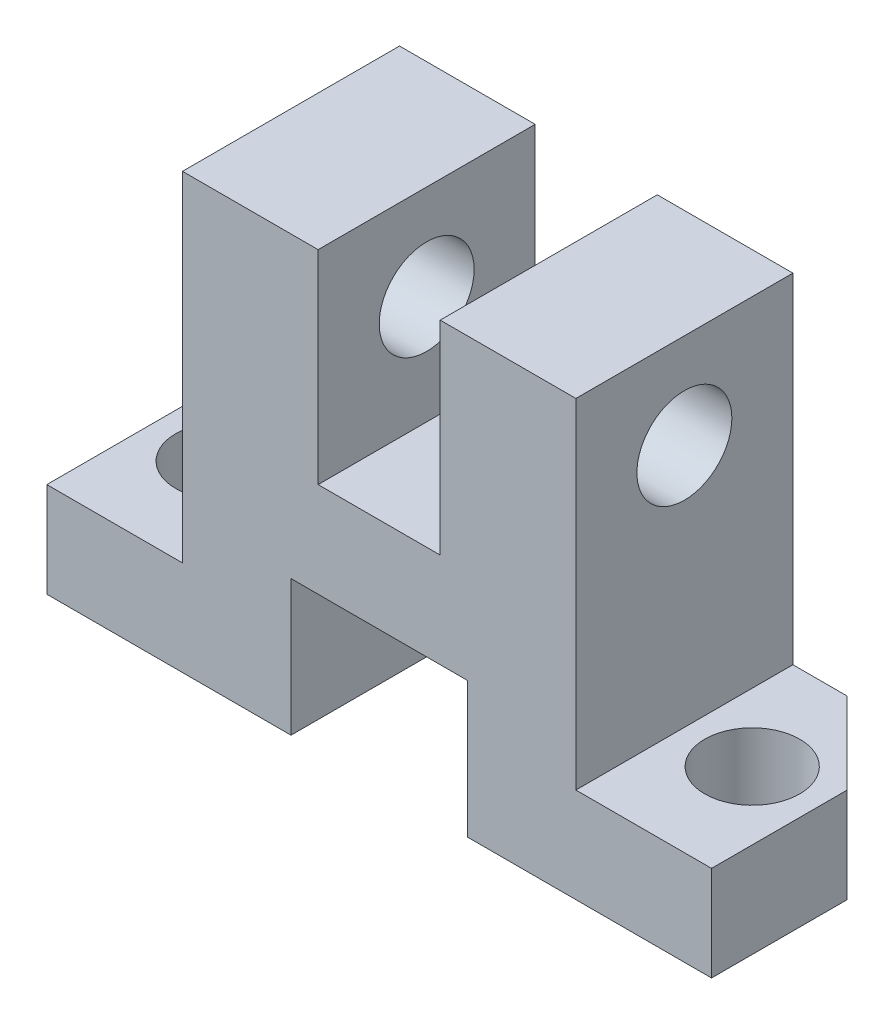
ISO-10303-21;
HEADER;
FILE_DESCRIPTION(('STEP AP214'),'2;1');
FILE_NAME('part.step','',(''),(''),'','','');
FILE_SCHEMA(('AUTOMOTIVE_DESIGN { 1 0 10303 214 1 1 1 1 }'));
ENDSEC;
DATA;
#1=APPLICATION_CONTEXT('core data for automotive mechanical design processes');
#2=APPLICATION_PROTOCOL_DEFINITION('international standard','automotive_design',2000,#1);
#3=PRODUCT_CONTEXT('',#1,'mechanical');
#4=PRODUCT('Part','Part','',(#3));
#5=PRODUCT_RELATED_PRODUCT_CATEGORY('part','',(#4));
#6=PRODUCT_DEFINITION_FORMATION('','',#4);
#7=PRODUCT_DEFINITION_CONTEXT('part definition',#1,'design');
#8=PRODUCT_DEFINITION('design','',#6,#7);
#9=PRODUCT_DEFINITION_SHAPE('','',#8);
#10=(LENGTH_UNIT() NAMED_UNIT(*) SI_UNIT(.MILLI.,.METRE.));
#11=(NAMED_UNIT(*) PLANE_ANGLE_UNIT() SI_UNIT($,.RADIAN.));
#12=(NAMED_UNIT(*) SI_UNIT($,.STERADIAN.) SOLID_ANGLE_UNIT());
#13=UNCERTAINTY_MEASURE_WITH_UNIT(LENGTH_MEASURE(1.E-05),#10,'distance_accuracy_value','');
#14=(GEOMETRIC_REPRESENTATION_CONTEXT(3) GLOBAL_UNCERTAINTY_ASSIGNED_CONTEXT((#13)) GLOBAL_UNIT_ASSIGNED_CONTEXT((#10,
#11,#12)) REPRESENTATION_CONTEXT('',''));
#15=CARTESIAN_POINT('',(0.,0.,0.));
#16=DIRECTION('',(0.,0.,1.));
#17=DIRECTION('',(1.,0.,0.));
#18=AXIS2_PLACEMENT_3D('',#15,#16,#17);
#19=CARTESIAN_POINT('',(14.5,-16.,16.));
#20=DIRECTION('',(-1.,0.,0.));
#21=DIRECTION('',(0.,0.,1.));
#22=AXIS2_PLACEMENT_3D('',#19,#20,#21);
#23=PLANE('',#22);
#24=CARTESIAN_POINT('',(14.5,9.,8.));
#25=DIRECTION('',(1.,0.,0.));
#26=DIRECTION('',(0.,0.,-1.));
#27=AXIS2_PLACEMENT_3D('',#24,#25,#26);
#28=CIRCLE('',#27,3.5);
#29=CARTESIAN_POINT('',(14.5,9.,4.5));
#30=VERTEX_POINT('',#29);
#31=EDGE_CURVE('E234',#30,#30,#28,.T.);
#32=ORIENTED_EDGE('',*,*,#31,.F.);
#33=EDGE_LOOP('',(#32));
#34=FACE_BOUND('',#33,.T.);
#35=DIRECTION('',(0.,0.,1.));
#36=VECTOR('',#35,1.);
#37=CARTESIAN_POINT('',(14.5,-9.00000000000001,0.));
#38=LINE('',#37,#36);
#39=CARTESIAN_POINT('',(14.5,-9.00000000000001,0.));
#40=VERTEX_POINT('',#39);
#41=CARTESIAN_POINT('',(14.5,-9.00000000000001,16.));
#42=VERTEX_POINT('',#41);
#43=EDGE_CURVE('E57',#40,#42,#38,.T.);
#44=ORIENTED_EDGE('',*,*,#43,.F.);
#45=DIRECTION('',(0.,1.,0.));
#46=VECTOR('',#45,1.);
#47=CARTESIAN_POINT('',(14.5,-16.,0.));
#48=LINE('',#47,#46);
#49=CARTESIAN_POINT('',(14.5,16.,0.));
#50=VERTEX_POINT('',#49);
#51=EDGE_CURVE('E287',#40,#50,#48,.T.);
#52=ORIENTED_EDGE('',*,*,#51,.T.);
#53=DIRECTION('',(0.,0.,-1.));
#54=VECTOR('',#53,1.);
#55=CARTESIAN_POINT('',(14.5,16.,16.));
#56=LINE('',#55,#54);
#57=CARTESIAN_POINT('',(14.5,16.,16.));
#58=VERTEX_POINT('',#57);
#59=EDGE_CURVE('E11',#58,#50,#56,.T.);
#60=ORIENTED_EDGE('',*,*,#59,.F.);
#61=DIRECTION('',(0.,1.,0.));
#62=VECTOR('',#61,1.);
#63=CARTESIAN_POINT('',(14.5,-16.,16.));
#64=LINE('',#63,#62);
#65=EDGE_CURVE('E291',#42,#58,#64,.T.);
#66=ORIENTED_EDGE('',*,*,#65,.F.);
#67=EDGE_LOOP('',(#44,#52,#60,#66));
#68=FACE_BOUND('',#67,.T.);
#69=ADVANCED_FACE('F41',(#34,#68),#23,.F.);
#70=CARTESIAN_POINT('',(-14.5,-16.,16.));
#71=DIRECTION('',(1.,0.,0.));
#72=DIRECTION('',(0.,0.,-1.));
#73=AXIS2_PLACEMENT_3D('',#70,#71,#72);
#74=PLANE('',#73);
#75=CARTESIAN_POINT('',(-14.5,9.,8.));
#76=DIRECTION('',(1.,0.,0.));
#77=DIRECTION('',(0.,0.,-1.));
#78=AXIS2_PLACEMENT_3D('',#75,#76,#77);
#79=CIRCLE('',#78,3.5);
#80=CARTESIAN_POINT('',(-14.5,9.,4.5));
#81=VERTEX_POINT('',#80);
#82=EDGE_CURVE('E232',#81,#81,#79,.T.);
#83=ORIENTED_EDGE('',*,*,#82,.T.);
#84=EDGE_LOOP('',(#83));
#85=FACE_BOUND('',#84,.T.);
#86=DIRECTION('',(0.,0.,-1.));
#87=VECTOR('',#86,1.);
#88=CARTESIAN_POINT('',(-14.5,-9.00000000000001,16.));
#89=LINE('',#88,#87);
#90=CARTESIAN_POINT('',(-14.5,-9.00000000000001,16.));
#91=VERTEX_POINT('',#90);
#92=CARTESIAN_POINT('',(-14.5,-9.00000000000001,0.));
#93=VERTEX_POINT('',#92);
#94=EDGE_CURVE('E226',#91,#93,#89,.T.);
#95=ORIENTED_EDGE('',*,*,#94,.F.);
#96=DIRECTION('',(0.,-1.,0.));
#97=VECTOR('',#96,1.);
#98=CARTESIAN_POINT('',(-14.5,-16.,16.));
#99=LINE('',#98,#97);
#100=CARTESIAN_POINT('',(-14.5,16.,16.));
#101=VERTEX_POINT('',#100);
#102=EDGE_CURVE('E297',#101,#91,#99,.T.);
#103=ORIENTED_EDGE('',*,*,#102,.F.);
#104=DIRECTION('',(0.,0.,-1.));
#105=VECTOR('',#104,1.);
#106=CARTESIAN_POINT('',(-14.5,16.,16.));
#107=LINE('',#106,#105);
#108=CARTESIAN_POINT('',(-14.5,16.,0.));
#109=VERTEX_POINT('',#108);
#110=EDGE_CURVE('E47',#101,#109,#107,.T.);
#111=ORIENTED_EDGE('',*,*,#110,.T.);
#112=DIRECTION('',(0.,-1.,0.));
#113=VECTOR('',#112,1.);
#114=CARTESIAN_POINT('',(-14.5,-16.,0.));
#115=LINE('',#114,#113);
#116=EDGE_CURVE('E315',#109,#93,#115,.T.);
#117=ORIENTED_EDGE('',*,*,#116,.T.);
#118=EDGE_LOOP('',(#95,#103,#111,#117));
#119=FACE_BOUND('',#118,.T.);
#120=ADVANCED_FACE('F321',(#85,#119),#74,.F.);
#121=CARTESIAN_POINT('',(-14.5,16.,16.));
#122=DIRECTION('',(0.,-1.,0.));
#123=DIRECTION('',(0.,0.,-1.));
#124=AXIS2_PLACEMENT_3D('',#121,#122,#123);
#125=PLANE('',#124);
#126=DIRECTION('',(-1.,0.,0.));
#127=VECTOR('',#126,1.);
#128=CARTESIAN_POINT('',(-14.5,16.,16.));
#129=LINE('',#128,#127);
#130=CARTESIAN_POINT('',(-4.5,16.,16.));
#131=VERTEX_POINT('',#130);
#132=EDGE_CURVE('E294',#131,#101,#129,.T.);
#133=ORIENTED_EDGE('',*,*,#132,.F.);
#134=DIRECTION('',(0.,0.,1.));
#135=VECTOR('',#134,1.);
#136=CARTESIAN_POINT('',(-4.5,16.,0.));
#137=LINE('',#136,#135);
#138=CARTESIAN_POINT('',(-4.5,16.,0.));
#139=VERTEX_POINT('',#138);
#140=EDGE_CURVE('E256',#139,#131,#137,.T.);
#141=ORIENTED_EDGE('',*,*,#140,.F.);
#142=DIRECTION('',(-1.,0.,0.));
#143=VECTOR('',#142,1.);
#144=CARTESIAN_POINT('',(-14.5,16.,0.));
#145=LINE('',#144,#143);
#146=EDGE_CURVE('E308',#139,#109,#145,.T.);
#147=ORIENTED_EDGE('',*,*,#146,.T.);
#148=ORIENTED_EDGE('',*,*,#110,.F.);
#149=EDGE_LOOP('',(#133,#141,#147,#148));
#150=FACE_BOUND('',#149,.T.);
#151=ADVANCED_FACE('F342',(#150),#125,.F.);
#152=CARTESIAN_POINT('',(-14.5,-16.,16.));
#153=DIRECTION('',(0.,1.,0.));
#154=DIRECTION('',(0.,0.,1.));
#155=AXIS2_PLACEMENT_3D('',#152,#153,#154);
#156=PLANE('',#155);
#157=CARTESIAN_POINT('',(19.5,-16.,8.));
#158=DIRECTION('',(0.,1.,0.));
#159=DIRECTION('',(0.,0.,1.));
#160=AXIS2_PLACEMENT_3D('',#157,#158,#159);
#161=CIRCLE('',#160,3.5);
#162=CARTESIAN_POINT('',(19.5,-16.,11.5));
#163=VERTEX_POINT('',#162);
#164=EDGE_CURVE('E554',#163,#163,#161,.T.);
#165=ORIENTED_EDGE('',*,*,#164,.T.);
#166=EDGE_LOOP('',(#165));
#167=FACE_BOUND('',#166,.T.);
#168=DIRECTION('',(1.,0.,0.));
#169=VECTOR('',#168,1.);
#170=CARTESIAN_POINT('',(-14.5,-16.,16.));
#171=LINE('',#170,#169);
#172=CARTESIAN_POINT('',(6.50000000000001,-16.,16.));
#173=VERTEX_POINT('',#172);
#174=CARTESIAN_POINT('',(24.5,-16.,16.));
#175=VERTEX_POINT('',#174);
#176=EDGE_CURVE('E303',#173,#175,#171,.T.);
#177=ORIENTED_EDGE('',*,*,#176,.F.);
#178=DIRECTION('',(0.,0.,1.));
#179=VECTOR('',#178,1.);
#180=CARTESIAN_POINT('',(6.50000000000001,-16.,0.));
#181=LINE('',#180,#179);
#182=CARTESIAN_POINT('',(6.50000000000001,-16.,0.));
#183=VERTEX_POINT('',#182);
#184=EDGE_CURVE('E282',#183,#173,#181,.T.);
#185=ORIENTED_EDGE('',*,*,#184,.F.);
#186=DIRECTION('',(1.,0.,0.));
#187=VECTOR('',#186,1.);
#188=CARTESIAN_POINT('',(-14.5,-16.,0.));
#189=LINE('',#188,#187);
#190=CARTESIAN_POINT('',(18.5,-16.,0.));
#191=VERTEX_POINT('',#190);
#192=EDGE_CURVE('E314',#183,#191,#189,.T.);
#193=ORIENTED_EDGE('',*,*,#192,.T.);
#194=DIRECTION('',(0.707106781186547,0.,0.707106781186548));
#195=VECTOR('',#194,1.);
#196=CARTESIAN_POINT('',(9.25,-16.,-9.25));
#197=LINE('',#196,#195);
#198=CARTESIAN_POINT('',(24.5,-16.,6.));
#199=VERTEX_POINT('',#198);
#200=EDGE_CURVE('E191',#191,#199,#197,.T.);
#201=ORIENTED_EDGE('',*,*,#200,.T.);
#202=DIRECTION('',(0.,0.,1.));
#203=VECTOR('',#202,1.);
#204=CARTESIAN_POINT('',(24.5,-16.,0.));
#205=LINE('',#204,#203);
#206=EDGE_CURVE('E175',#199,#175,#205,.T.);
#207=ORIENTED_EDGE('',*,*,#206,.T.);
#208=EDGE_LOOP('',(#177,#185,#193,#201,#207));
#209=FACE_BOUND('',#208,.T.);
#210=ADVANCED_FACE('F357',(#167,#209),#156,.F.);
#211=CARTESIAN_POINT('',(4.5,16.,0.));
#212=VERTEX_POINT('',#211);
#213=EDGE_CURVE('E307',#50,#212,#145,.T.);
#214=ORIENTED_EDGE('',*,*,#213,.T.);
#215=DIRECTION('',(0.,0.,1.));
#216=VECTOR('',#215,1.);
#217=CARTESIAN_POINT('',(4.5,16.,0.));
#218=LINE('',#217,#216);
#219=CARTESIAN_POINT('',(4.5,16.,16.));
#220=VERTEX_POINT('',#219);
#221=EDGE_CURVE('E265',#212,#220,#218,.T.);
#222=ORIENTED_EDGE('',*,*,#221,.T.);
#223=EDGE_CURVE('E300',#58,#220,#129,.T.);
#224=ORIENTED_EDGE('',*,*,#223,.F.);
#225=ORIENTED_EDGE('',*,*,#59,.T.);
#226=EDGE_LOOP('',(#214,#222,#224,#225));
#227=FACE_BOUND('',#226,.T.);
#228=ADVANCED_FACE('F354',(#227),#125,.F.);
#229=CARTESIAN_POINT('',(-19.5,-16.,8.));
#230=DIRECTION('',(0.,1.,0.));
#231=DIRECTION('',(0.,0.,1.));
#232=AXIS2_PLACEMENT_3D('',#229,#230,#231);
#233=CIRCLE('',#232,3.5);
#234=CARTESIAN_POINT('',(-19.5,-16.,11.5));
#235=VERTEX_POINT('',#234);
#236=EDGE_CURVE('E205',#235,#235,#233,.T.);
#237=ORIENTED_EDGE('',*,*,#236,.T.);
#238=EDGE_LOOP('',(#237));
#239=FACE_BOUND('',#238,.T.);
#240=CARTESIAN_POINT('',(-18.5,-16.,0.));
#241=VERTEX_POINT('',#240);
#242=CARTESIAN_POINT('',(-6.5,-16.,0.));
#243=VERTEX_POINT('',#242);
#244=EDGE_CURVE('E298',#241,#243,#189,.T.);
#245=ORIENTED_EDGE('',*,*,#244,.T.);
#246=DIRECTION('',(0.,0.,1.));
#247=VECTOR('',#246,1.);
#248=CARTESIAN_POINT('',(-6.5,-16.,0.));
#249=LINE('',#248,#247);
#250=CARTESIAN_POINT('',(-6.5,-16.,16.));
#251=VERTEX_POINT('',#250);
#252=EDGE_CURVE('E289',#243,#251,#249,.T.);
#253=ORIENTED_EDGE('',*,*,#252,.T.);
#254=CARTESIAN_POINT('',(-24.5,-16.,16.));
#255=VERTEX_POINT('',#254);
#256=EDGE_CURVE('E302',#255,#251,#171,.T.);
#257=ORIENTED_EDGE('',*,*,#256,.F.);
#258=DIRECTION('',(0.,0.,-1.));
#259=VECTOR('',#258,1.);
#260=CARTESIAN_POINT('',(-24.5,-16.,6.));
#261=LINE('',#260,#259);
#262=CARTESIAN_POINT('',(-24.5,-16.,6.));
#263=VERTEX_POINT('',#262);
#264=EDGE_CURVE('E207',#255,#263,#261,.T.);
#265=ORIENTED_EDGE('',*,*,#264,.T.);
#266=DIRECTION('',(0.707106781186547,0.,-0.707106781186548));
#267=VECTOR('',#266,1.);
#268=CARTESIAN_POINT('',(-18.5,-16.,0.));
#269=LINE('',#268,#267);
#270=EDGE_CURVE('E215',#263,#241,#269,.T.);
#271=ORIENTED_EDGE('',*,*,#270,.T.);
#272=EDGE_LOOP('',(#245,#253,#257,#265,#271));
#273=FACE_BOUND('',#272,.T.);
#274=ADVANCED_FACE('F375',(#239,#273),#156,.F.);
#275=CARTESIAN_POINT('',(0.,0.,16.));
#276=DIRECTION('',(0.,0.,-1.));
#277=DIRECTION('',(-1.,0.,0.));
#278=AXIS2_PLACEMENT_3D('',#275,#276,#277);
#279=PLANE('',#278);
#280=ORIENTED_EDGE('',*,*,#256,.T.);
#281=DIRECTION('',(0.,-1.,0.));
#282=VECTOR('',#281,1.);
#283=CARTESIAN_POINT('',(-6.5,-16.,16.));
#284=LINE('',#283,#282);
#285=CARTESIAN_POINT('',(-6.5,-6.,16.));
#286=VERTEX_POINT('',#285);
#287=EDGE_CURVE('E275',#286,#251,#284,.T.);
#288=ORIENTED_EDGE('',*,*,#287,.F.);
#289=DIRECTION('',(-1.,0.,0.));
#290=VECTOR('',#289,1.);
#291=CARTESIAN_POINT('',(-6.5,-6.,16.));
#292=LINE('',#291,#290);
#293=CARTESIAN_POINT('',(6.5,-6.00000000000001,16.));
#294=VERTEX_POINT('',#293);
#295=EDGE_CURVE('E278',#294,#286,#292,.T.);
#296=ORIENTED_EDGE('',*,*,#295,.F.);
#297=DIRECTION('',(0.,1.,0.));
#298=VECTOR('',#297,1.);
#299=CARTESIAN_POINT('',(6.50000000000001,-16.,16.));
#300=LINE('',#299,#298);
#301=EDGE_CURVE('E261',#173,#294,#300,.T.);
#302=ORIENTED_EDGE('',*,*,#301,.F.);
#303=ORIENTED_EDGE('',*,*,#176,.T.);
#304=DIRECTION('',(0.,-1.,0.));
#305=VECTOR('',#304,1.);
#306=CARTESIAN_POINT('',(24.5,-9.00000000000001,16.));
#307=LINE('',#306,#305);
#308=CARTESIAN_POINT('',(24.5,-9.00000000000001,16.));
#309=VERTEX_POINT('',#308);
#310=EDGE_CURVE('E180',#309,#175,#307,.T.);
#311=ORIENTED_EDGE('',*,*,#310,.F.);
#312=DIRECTION('',(1.,0.,0.));
#313=VECTOR('',#312,1.);
#314=CARTESIAN_POINT('',(0.,-9.00000000000001,16.));
#315=LINE('',#314,#313);
#316=EDGE_CURVE('E190',#42,#309,#315,.T.);
#317=ORIENTED_EDGE('',*,*,#316,.F.);
#318=ORIENTED_EDGE('',*,*,#65,.T.);
#319=ORIENTED_EDGE('',*,*,#223,.T.);
#320=DIRECTION('',(0.,1.,0.));
#321=VECTOR('',#320,1.);
#322=CARTESIAN_POINT('',(4.5,16.,16.));
#323=LINE('',#322,#321);
#324=CARTESIAN_POINT('',(4.5,0.999999999999997,16.));
#325=VERTEX_POINT('',#324);
#326=EDGE_CURVE('E247',#325,#220,#323,.T.);
#327=ORIENTED_EDGE('',*,*,#326,.F.);
#328=DIRECTION('',(1.,0.,0.));
#329=VECTOR('',#328,1.);
#330=CARTESIAN_POINT('',(-4.5,0.999999999999997,16.));
#331=LINE('',#330,#329);
#332=CARTESIAN_POINT('',(-4.5,0.999999999999997,16.));
#333=VERTEX_POINT('',#332);
#334=EDGE_CURVE('E253',#333,#325,#331,.T.);
#335=ORIENTED_EDGE('',*,*,#334,.F.);
#336=DIRECTION('',(0.,-1.,0.));
#337=VECTOR('',#336,1.);
#338=CARTESIAN_POINT('',(-4.5,16.,16.));
#339=LINE('',#338,#337);
#340=EDGE_CURVE('E243',#131,#333,#339,.T.);
#341=ORIENTED_EDGE('',*,*,#340,.F.);
#342=ORIENTED_EDGE('',*,*,#132,.T.);
#343=ORIENTED_EDGE('',*,*,#102,.T.);
#344=DIRECTION('',(-1.,0.,0.));
#345=VECTOR('',#344,1.);
#346=CARTESIAN_POINT('',(-6.5,-9.00000000000001,16.));
#347=LINE('',#346,#345);
#348=CARTESIAN_POINT('',(-24.5,-9.00000000000001,16.));
#349=VERTEX_POINT('',#348);
#350=EDGE_CURVE('E212',#91,#349,#347,.T.);
#351=ORIENTED_EDGE('',*,*,#350,.T.);
#352=DIRECTION('',(0.,-1.,0.));
#353=VECTOR('',#352,1.);
#354=CARTESIAN_POINT('',(-24.5,-9.00000000000001,16.));
#355=LINE('',#354,#353);
#356=EDGE_CURVE('E219',#349,#255,#355,.T.);
#357=ORIENTED_EDGE('',*,*,#356,.T.);
#358=EDGE_LOOP('',(#280,#288,#296,#302,#303,#311,#317,#318,#319,#327,#335,#341,#342,#343,#351,#357));
#359=FACE_BOUND('',#358,.T.);
#360=ADVANCED_FACE('F337',(#359),#279,.F.);
#361=CARTESIAN_POINT('',(0.,0.,0.));
#362=DIRECTION('',(0.,0.,-1.));
#363=DIRECTION('',(-1.,0.,0.));
#364=AXIS2_PLACEMENT_3D('',#361,#362,#363);
#365=PLANE('',#364);
#366=ORIENTED_EDGE('',*,*,#244,.F.);
#367=DIRECTION('',(0.,-1.,0.));
#368=VECTOR('',#367,1.);
#369=CARTESIAN_POINT('',(-18.5,-9.00000000000001,0.));
#370=LINE('',#369,#368);
#371=CARTESIAN_POINT('',(-18.5,-9.00000000000001,0.));
#372=VERTEX_POINT('',#371);
#373=EDGE_CURVE('E223',#372,#241,#370,.T.);
#374=ORIENTED_EDGE('',*,*,#373,.F.);
#375=DIRECTION('',(1.,0.,0.));
#376=VECTOR('',#375,1.);
#377=CARTESIAN_POINT('',(-14.5,-9.00000000000001,0.));
#378=LINE('',#377,#376);
#379=EDGE_CURVE('E206',#372,#93,#378,.T.);
#380=ORIENTED_EDGE('',*,*,#379,.T.);
#381=ORIENTED_EDGE('',*,*,#116,.F.);
#382=ORIENTED_EDGE('',*,*,#146,.F.);
#383=DIRECTION('',(0.,-1.,0.));
#384=VECTOR('',#383,1.);
#385=CARTESIAN_POINT('',(-4.5,16.,0.));
#386=LINE('',#385,#384);
#387=CARTESIAN_POINT('',(-4.5,0.999999999999997,0.));
#388=VERTEX_POINT('',#387);
#389=EDGE_CURVE('E242',#139,#388,#386,.T.);
#390=ORIENTED_EDGE('',*,*,#389,.T.);
#391=DIRECTION('',(1.,0.,0.));
#392=VECTOR('',#391,1.);
#393=CARTESIAN_POINT('',(-4.5,0.999999999999997,0.));
#394=LINE('',#393,#392);
#395=CARTESIAN_POINT('',(4.5,0.999999999999997,0.));
#396=VERTEX_POINT('',#395);
#397=EDGE_CURVE('E250',#388,#396,#394,.T.);
#398=ORIENTED_EDGE('',*,*,#397,.T.);
#399=DIRECTION('',(0.,1.,0.));
#400=VECTOR('',#399,1.);
#401=CARTESIAN_POINT('',(4.5,16.,0.));
#402=LINE('',#401,#400);
#403=EDGE_CURVE('E61',#396,#212,#402,.T.);
#404=ORIENTED_EDGE('',*,*,#403,.T.);
#405=ORIENTED_EDGE('',*,*,#213,.F.);
#406=ORIENTED_EDGE('',*,*,#51,.F.);
#407=DIRECTION('',(1.,0.,0.));
#408=VECTOR('',#407,1.);
#409=CARTESIAN_POINT('',(0.,-9.00000000000001,0.));
#410=LINE('',#409,#408);
#411=CARTESIAN_POINT('',(18.5,-9.00000000000001,0.));
#412=VERTEX_POINT('',#411);
#413=EDGE_CURVE('E178',#40,#412,#410,.T.);
#414=ORIENTED_EDGE('',*,*,#413,.T.);
#415=DIRECTION('',(0.,-1.,0.));
#416=VECTOR('',#415,1.);
#417=CARTESIAN_POINT('',(18.5,-9.00000000000001,0.));
#418=LINE('',#417,#416);
#419=EDGE_CURVE('E195',#412,#191,#418,.T.);
#420=ORIENTED_EDGE('',*,*,#419,.T.);
#421=ORIENTED_EDGE('',*,*,#192,.F.);
#422=DIRECTION('',(0.,1.,0.));
#423=VECTOR('',#422,1.);
#424=CARTESIAN_POINT('',(6.50000000000001,-16.,0.));
#425=LINE('',#424,#423);
#426=CARTESIAN_POINT('',(6.5,-6.00000000000001,0.));
#427=VERTEX_POINT('',#426);
#428=EDGE_CURVE('E270',#183,#427,#425,.T.);
#429=ORIENTED_EDGE('',*,*,#428,.T.);
#430=DIRECTION('',(-1.,0.,0.));
#431=VECTOR('',#430,1.);
#432=CARTESIAN_POINT('',(-6.5,-6.,0.));
#433=LINE('',#432,#431);
#434=CARTESIAN_POINT('',(-6.5,-6.,0.));
#435=VERTEX_POINT('',#434);
#436=EDGE_CURVE('E272',#427,#435,#433,.T.);
#437=ORIENTED_EDGE('',*,*,#436,.T.);
#438=DIRECTION('',(0.,-1.,0.));
#439=VECTOR('',#438,1.);
#440=CARTESIAN_POINT('',(-6.5,-16.,0.));
#441=LINE('',#440,#439);
#442=EDGE_CURVE('E273',#435,#243,#441,.T.);
#443=ORIENTED_EDGE('',*,*,#442,.T.);
#444=EDGE_LOOP('',(#366,#374,#380,#381,#382,#390,#398,#404,#405,#406,#414,#420,#421,#429,#437,#443));
#445=FACE_BOUND('',#444,.T.);
#446=ADVANCED_FACE('F327',(#445),#365,.T.);
#447=CARTESIAN_POINT('',(6.50000000000001,-16.,0.));
#448=DIRECTION('',(1.,0.,0.));
#449=DIRECTION('',(0.,1.,0.));
#450=AXIS2_PLACEMENT_3D('',#447,#448,#449);
#451=PLANE('',#450);
#452=ORIENTED_EDGE('',*,*,#301,.T.);
#453=DIRECTION('',(0.,0.,1.));
#454=VECTOR('',#453,1.);
#455=CARTESIAN_POINT('',(6.5,-6.00000000000001,0.));
#456=LINE('',#455,#454);
#457=EDGE_CURVE('E280',#427,#294,#456,.T.);
#458=ORIENTED_EDGE('',*,*,#457,.F.);
#459=ORIENTED_EDGE('',*,*,#428,.F.);
#460=ORIENTED_EDGE('',*,*,#184,.T.);
#461=EDGE_LOOP('',(#452,#458,#459,#460));
#462=FACE_BOUND('',#461,.T.);
#463=ADVANCED_FACE('F363',(#462),#451,.F.);
#464=CARTESIAN_POINT('',(-6.5,-16.,0.));
#465=DIRECTION('',(-1.,0.,0.));
#466=DIRECTION('',(0.,0.,1.));
#467=AXIS2_PLACEMENT_3D('',#464,#465,#466);
#468=PLANE('',#467);
#469=ORIENTED_EDGE('',*,*,#252,.F.);
#470=ORIENTED_EDGE('',*,*,#442,.F.);
#471=DIRECTION('',(0.,0.,1.));
#472=VECTOR('',#471,1.);
#473=CARTESIAN_POINT('',(-6.5,-6.,0.));
#474=LINE('',#473,#472);
#475=EDGE_CURVE('E288',#435,#286,#474,.T.);
#476=ORIENTED_EDGE('',*,*,#475,.T.);
#477=ORIENTED_EDGE('',*,*,#287,.T.);
#478=EDGE_LOOP('',(#469,#470,#476,#477));
#479=FACE_BOUND('',#478,.T.);
#480=ADVANCED_FACE('F369',(#479),#468,.F.);
#481=CARTESIAN_POINT('',(-6.5,-6.,0.));
#482=DIRECTION('',(0.,1.,0.));
#483=DIRECTION('',(-1.,0.,0.));
#484=AXIS2_PLACEMENT_3D('',#481,#482,#483);
#485=PLANE('',#484);
#486=ORIENTED_EDGE('',*,*,#295,.T.);
#487=ORIENTED_EDGE('',*,*,#475,.F.);
#488=ORIENTED_EDGE('',*,*,#436,.F.);
#489=ORIENTED_EDGE('',*,*,#457,.T.);
#490=EDGE_LOOP('',(#486,#487,#488,#489));
#491=FACE_BOUND('',#490,.T.);
#492=ADVANCED_FACE('F366',(#491),#485,.F.);
#493=CARTESIAN_POINT('',(-4.5,16.,0.));
#494=DIRECTION('',(-1.,0.,0.));
#495=DIRECTION('',(0.,-1.,0.));
#496=AXIS2_PLACEMENT_3D('',#493,#494,#495);
#497=PLANE('',#496);
#498=CARTESIAN_POINT('',(-4.5,9.,8.));
#499=DIRECTION('',(-1.,0.,0.));
#500=DIRECTION('',(0.,-1.,0.));
#501=AXIS2_PLACEMENT_3D('',#498,#499,#500);
#502=CIRCLE('',#501,3.5);
#503=CARTESIAN_POINT('',(-4.5,9.,4.5));
#504=VERTEX_POINT('',#503);
#505=EDGE_CURVE('E239',#504,#504,#502,.T.);
#506=ORIENTED_EDGE('',*,*,#505,.T.);
#507=EDGE_LOOP('',(#506));
#508=FACE_BOUND('',#507,.T.);
#509=ORIENTED_EDGE('',*,*,#340,.T.);
#510=DIRECTION('',(0.,0.,1.));
#511=VECTOR('',#510,1.);
#512=CARTESIAN_POINT('',(-4.5,0.999999999999997,0.));
#513=LINE('',#512,#511);
#514=EDGE_CURVE('E255',#388,#333,#513,.T.);
#515=ORIENTED_EDGE('',*,*,#514,.F.);
#516=ORIENTED_EDGE('',*,*,#389,.F.);
#517=ORIENTED_EDGE('',*,*,#140,.T.);
#518=EDGE_LOOP('',(#509,#515,#516,#517));
#519=FACE_BOUND('',#518,.T.);
#520=ADVANCED_FACE('F344',(#508,#519),#497,.F.);
#521=CARTESIAN_POINT('',(4.5,16.,0.));
#522=DIRECTION('',(1.,0.,0.));
#523=DIRECTION('',(0.,1.,0.));
#524=AXIS2_PLACEMENT_3D('',#521,#522,#523);
#525=PLANE('',#524);
#526=CARTESIAN_POINT('',(4.5,9.,8.));
#527=DIRECTION('',(1.,0.,0.));
#528=DIRECTION('',(0.,1.,0.));
#529=AXIS2_PLACEMENT_3D('',#526,#527,#528);
#530=CIRCLE('',#529,3.5);
#531=CARTESIAN_POINT('',(4.5,9.,4.5));
#532=VERTEX_POINT('',#531);
#533=EDGE_CURVE('E42',#532,#532,#530,.T.);
#534=ORIENTED_EDGE('',*,*,#533,.T.);
#535=EDGE_LOOP('',(#534));
#536=FACE_BOUND('',#535,.T.);
#537=ORIENTED_EDGE('',*,*,#326,.T.);
#538=ORIENTED_EDGE('',*,*,#221,.F.);
#539=ORIENTED_EDGE('',*,*,#403,.F.);
#540=DIRECTION('',(0.,0.,1.));
#541=VECTOR('',#540,1.);
#542=CARTESIAN_POINT('',(4.5,0.999999999999997,0.));
#543=LINE('',#542,#541);
#544=EDGE_CURVE('E264',#396,#325,#543,.T.);
#545=ORIENTED_EDGE('',*,*,#544,.T.);
#546=EDGE_LOOP('',(#537,#538,#539,#545));
#547=FACE_BOUND('',#546,.T.);
#548=ADVANCED_FACE('F347',(#536,#547),#525,.F.);
#549=CARTESIAN_POINT('',(-4.5,0.999999999999997,0.));
#550=DIRECTION('',(0.,-1.,0.));
#551=DIRECTION('',(0.,0.,-1.));
#552=AXIS2_PLACEMENT_3D('',#549,#550,#551);
#553=PLANE('',#552);
#554=ORIENTED_EDGE('',*,*,#334,.T.);
#555=ORIENTED_EDGE('',*,*,#544,.F.);
#556=ORIENTED_EDGE('',*,*,#397,.F.);
#557=ORIENTED_EDGE('',*,*,#514,.T.);
#558=EDGE_LOOP('',(#554,#555,#556,#557));
#559=FACE_BOUND('',#558,.T.);
#560=ADVANCED_FACE('F350',(#559),#553,.F.);
#561=CARTESIAN_POINT('',(-14.5,9.,8.));
#562=DIRECTION('',(1.,0.,0.));
#563=DIRECTION('',(0.,0.,-1.));
#564=AXIS2_PLACEMENT_3D('',#561,#562,#563);
#565=CYLINDRICAL_SURFACE('',#564,3.5);
#566=CARTESIAN_POINT('',(14.5,9.,4.5));
#567=CARTESIAN_POINT('',(14.3958333333333,9.,4.5));
#568=CARTESIAN_POINT('',(14.2916666666667,9.,4.5));
#569=CARTESIAN_POINT('',(14.0833333333333,9.,4.5));
#570=CARTESIAN_POINT('',(13.9791666666667,9.,4.5));
#571=CARTESIAN_POINT('',(13.7708333333333,9.,4.5));
#572=CARTESIAN_POINT('',(13.6666666666667,9.,4.5));
#573=CARTESIAN_POINT('',(13.4583333333333,9.,4.5));
#574=CARTESIAN_POINT('',(13.3541666666667,9.,4.5));
#575=CARTESIAN_POINT('',(13.1458333333333,9.,4.5));
#576=CARTESIAN_POINT('',(13.0416666666667,9.,4.5));
#577=CARTESIAN_POINT('',(12.8333333333333,9.,4.5));
#578=CARTESIAN_POINT('',(12.7291666666667,9.,4.5));
#579=CARTESIAN_POINT('',(12.5208333333333,9.,4.5));
#580=CARTESIAN_POINT('',(12.4166666666667,9.,4.5));
#581=CARTESIAN_POINT('',(12.2083333333333,9.,4.5));
#582=CARTESIAN_POINT('',(12.1041666666667,9.,4.5));
#583=CARTESIAN_POINT('',(11.8958333333333,9.,4.5));
#584=CARTESIAN_POINT('',(11.7916666666667,9.,4.5));
#585=CARTESIAN_POINT('',(11.5833333333333,9.,4.5));
#586=CARTESIAN_POINT('',(11.4791666666667,9.,4.5));
#587=CARTESIAN_POINT('',(11.2708333333333,9.,4.5));
#588=CARTESIAN_POINT('',(11.1666666666667,9.,4.5));
#589=CARTESIAN_POINT('',(10.9583333333333,9.,4.5));
#590=CARTESIAN_POINT('',(10.8541666666667,9.,4.5));
#591=CARTESIAN_POINT('',(10.6458333333333,9.,4.5));
#592=CARTESIAN_POINT('',(10.5416666666667,9.,4.5));
#593=CARTESIAN_POINT('',(10.3333333333333,9.,4.5));
#594=CARTESIAN_POINT('',(10.2291666666667,9.,4.5));
#595=CARTESIAN_POINT('',(10.0208333333333,9.,4.5));
#596=CARTESIAN_POINT('',(9.91666666666667,9.,4.5));
#597=CARTESIAN_POINT('',(9.70833333333333,9.,4.5));
#598=CARTESIAN_POINT('',(9.60416666666667,9.,4.5));
#599=CARTESIAN_POINT('',(9.39583333333333,9.,4.5));
#600=CARTESIAN_POINT('',(9.29166666666666,9.,4.5));
#601=CARTESIAN_POINT('',(9.08333333333333,9.,4.5));
#602=CARTESIAN_POINT('',(8.97916666666666,9.,4.5));
#603=CARTESIAN_POINT('',(8.77083333333333,9.,4.5));
#604=CARTESIAN_POINT('',(8.66666666666666,9.,4.5));
#605=CARTESIAN_POINT('',(8.45833333333333,9.,4.5));
#606=CARTESIAN_POINT('',(8.35416666666666,9.,4.5));
#607=CARTESIAN_POINT('',(8.14583333333333,9.,4.5));
#608=CARTESIAN_POINT('',(8.04166666666666,9.,4.5));
#609=CARTESIAN_POINT('',(7.83333333333333,9.,4.5));
#610=CARTESIAN_POINT('',(7.72916666666667,9.,4.5));
#611=CARTESIAN_POINT('',(7.52083333333333,9.,4.5));
#612=CARTESIAN_POINT('',(7.41666666666667,9.,4.5));
#613=CARTESIAN_POINT('',(7.20833333333333,9.,4.5));
#614=CARTESIAN_POINT('',(7.10416666666667,9.,4.5));
#615=CARTESIAN_POINT('',(6.89583333333333,9.,4.5));
#616=CARTESIAN_POINT('',(6.79166666666667,9.,4.5));
#617=CARTESIAN_POINT('',(6.58333333333333,9.,4.5));
#618=CARTESIAN_POINT('',(6.47916666666667,9.,4.5));
#619=CARTESIAN_POINT('',(6.27083333333333,9.,4.5));
#620=CARTESIAN_POINT('',(6.16666666666667,9.,4.5));
#621=CARTESIAN_POINT('',(5.95833333333334,9.,4.5));
#622=CARTESIAN_POINT('',(5.85416666666667,9.,4.5));
#623=CARTESIAN_POINT('',(5.64583333333333,9.,4.5));
#624=CARTESIAN_POINT('',(5.54166666666667,9.,4.5));
#625=CARTESIAN_POINT('',(5.33333333333333,9.,4.5));
#626=CARTESIAN_POINT('',(5.22916666666667,9.,4.5));
#627=CARTESIAN_POINT('',(5.02083333333333,9.,4.5));
#628=CARTESIAN_POINT('',(4.91666666666667,9.,4.5));
#629=CARTESIAN_POINT('',(4.70833333333333,9.,4.5));
#630=CARTESIAN_POINT('',(4.60416666666667,9.,4.5));
#631=CARTESIAN_POINT('',(4.5,9.,4.5));
#632=B_SPLINE_CURVE_WITH_KNOTS('',3,(#566,#567,#568,#569,#570,#571,#572,#573,#574,#575,#576,
#577,#578,#579,#580,#581,#582,#583,#584,#585,#586,#587,#588,#589,#590,#591,#592,#593,#594,#595,
#596,#597,#598,#599,#600,#601,#602,#603,#604,#605,#606,#607,#608,#609,#610,#611,#612,#613,#614,
#615,#616,#617,#618,#619,#620,#621,#622,#623,#624,#625,#626,#627,#628,#629,#630,#631),
.UNSPECIFIED.,.F.,.F.,(4,2,2,2,2,2,2,2,2,2,2,2,2,2,2,2,2,2,2,2,2,2,2,2,2,2,2,2,2,2,2,2,4),(0.,
0.3125,0.625000000000001,0.937500000000001,1.25,1.5625,1.875,2.1875,2.5,2.8125,3.125,3.4375,
3.75,4.0625,4.375,4.6875,5.,5.3125,5.625,5.9375,6.25,6.5625,6.875,7.1875,7.5,7.8125,8.125,
8.43749999999999,8.74999999999999,9.06249999999999,9.37499999999999,9.68749999999999,
9.99999999999999),.UNSPECIFIED.);
#633=EDGE_CURVE('BSEAM400',#30,#532,#632,.T.);
#634=ORIENTED_EDGE('',*,*,#31,.T.);
#635=ORIENTED_EDGE('',*,*,#533,.F.);
#636=ORIENTED_EDGE('',*,*,#633,.T.);
#637=ORIENTED_EDGE('',*,*,#633,.F.);
#638=EDGE_LOOP('',(#634,#636,#635,#637));
#639=FACE_BOUND('',#638,.T.);
#640=ADVANCED_FACE('F400',(#639),#565,.F.);
#641=CARTESIAN_POINT('',(-14.5,9.,4.5));
#642=CARTESIAN_POINT('',(-14.3958333333333,9.,4.5));
#643=CARTESIAN_POINT('',(-14.2916666666667,9.,4.5));
#644=CARTESIAN_POINT('',(-14.0833333333333,9.,4.5));
#645=CARTESIAN_POINT('',(-13.9791666666667,9.,4.5));
#646=CARTESIAN_POINT('',(-13.7708333333333,9.,4.5));
#647=CARTESIAN_POINT('',(-13.6666666666667,9.,4.5));
#648=CARTESIAN_POINT('',(-13.4583333333333,9.,4.5));
#649=CARTESIAN_POINT('',(-13.3541666666667,9.,4.5));
#650=CARTESIAN_POINT('',(-13.1458333333333,9.,4.5));
#651=CARTESIAN_POINT('',(-13.0416666666667,9.,4.5));
#652=CARTESIAN_POINT('',(-12.8333333333333,9.,4.5));
#653=CARTESIAN_POINT('',(-12.7291666666667,9.,4.5));
#654=CARTESIAN_POINT('',(-12.5208333333333,9.,4.5));
#655=CARTESIAN_POINT('',(-12.4166666666667,9.,4.5));
#656=CARTESIAN_POINT('',(-12.2083333333333,9.,4.5));
#657=CARTESIAN_POINT('',(-12.1041666666667,9.,4.5));
#658=CARTESIAN_POINT('',(-11.8958333333333,9.,4.5));
#659=CARTESIAN_POINT('',(-11.7916666666667,9.,4.5));
#660=CARTESIAN_POINT('',(-11.5833333333333,9.,4.5));
#661=CARTESIAN_POINT('',(-11.4791666666667,9.,4.5));
#662=CARTESIAN_POINT('',(-11.2708333333333,9.,4.5));
#663=CARTESIAN_POINT('',(-11.1666666666667,9.,4.5));
#664=CARTESIAN_POINT('',(-10.9583333333333,9.,4.5));
#665=CARTESIAN_POINT('',(-10.8541666666667,9.,4.5));
#666=CARTESIAN_POINT('',(-10.6458333333333,9.,4.5));
#667=CARTESIAN_POINT('',(-10.5416666666667,9.,4.5));
#668=CARTESIAN_POINT('',(-10.3333333333333,9.,4.5));
#669=CARTESIAN_POINT('',(-10.2291666666667,9.,4.5));
#670=CARTESIAN_POINT('',(-10.0208333333333,9.,4.5));
#671=CARTESIAN_POINT('',(-9.91666666666667,9.,4.5));
#672=CARTESIAN_POINT('',(-9.70833333333333,9.,4.5));
#673=CARTESIAN_POINT('',(-9.60416666666667,9.,4.5));
#674=CARTESIAN_POINT('',(-9.39583333333333,9.,4.5));
#675=CARTESIAN_POINT('',(-9.29166666666667,9.,4.5));
#676=CARTESIAN_POINT('',(-9.08333333333333,9.,4.5));
#677=CARTESIAN_POINT('',(-8.97916666666667,9.,4.5));
#678=CARTESIAN_POINT('',(-8.77083333333333,9.,4.5));
#679=CARTESIAN_POINT('',(-8.66666666666667,9.,4.5));
#680=CARTESIAN_POINT('',(-8.45833333333333,9.,4.5));
#681=CARTESIAN_POINT('',(-8.35416666666667,9.,4.5));
#682=CARTESIAN_POINT('',(-8.14583333333333,9.,4.5));
#683=CARTESIAN_POINT('',(-8.04166666666667,9.,4.5));
#684=CARTESIAN_POINT('',(-7.83333333333333,9.,4.5));
#685=CARTESIAN_POINT('',(-7.72916666666667,9.,4.5));
#686=CARTESIAN_POINT('',(-7.52083333333333,9.,4.5));
#687=CARTESIAN_POINT('',(-7.41666666666667,9.,4.5));
#688=CARTESIAN_POINT('',(-7.20833333333333,9.,4.5));
#689=CARTESIAN_POINT('',(-7.10416666666667,9.,4.5));
#690=CARTESIAN_POINT('',(-6.89583333333333,9.,4.5));
#691=CARTESIAN_POINT('',(-6.79166666666667,9.,4.5));
#692=CARTESIAN_POINT('',(-6.58333333333333,9.,4.5));
#693=CARTESIAN_POINT('',(-6.47916666666667,9.,4.5));
#694=CARTESIAN_POINT('',(-6.27083333333333,9.,4.5));
#695=CARTESIAN_POINT('',(-6.16666666666667,9.,4.5));
#696=CARTESIAN_POINT('',(-5.95833333333333,9.,4.5));
#697=CARTESIAN_POINT('',(-5.85416666666667,9.,4.5));
#698=CARTESIAN_POINT('',(-5.64583333333333,9.,4.5));
#699=CARTESIAN_POINT('',(-5.54166666666667,9.,4.5));
#700=CARTESIAN_POINT('',(-5.33333333333333,9.,4.5));
#701=CARTESIAN_POINT('',(-5.22916666666667,9.,4.5));
#702=CARTESIAN_POINT('',(-5.02083333333333,9.,4.5));
#703=CARTESIAN_POINT('',(-4.91666666666667,9.,4.5));
#704=CARTESIAN_POINT('',(-4.70833333333333,9.,4.5));
#705=CARTESIAN_POINT('',(-4.60416666666667,9.,4.5));
#706=CARTESIAN_POINT('',(-4.5,9.,4.5));
#707=B_SPLINE_CURVE_WITH_KNOTS('',3,(#641,#642,#643,#644,#645,#646,#647,#648,#649,#650,#651,
#652,#653,#654,#655,#656,#657,#658,#659,#660,#661,#662,#663,#664,#665,#666,#667,#668,#669,#670,
#671,#672,#673,#674,#675,#676,#677,#678,#679,#680,#681,#682,#683,#684,#685,#686,#687,#688,#689,
#690,#691,#692,#693,#694,#695,#696,#697,#698,#699,#700,#701,#702,#703,#704,#705,#706),
.UNSPECIFIED.,.F.,.F.,(4,2,2,2,2,2,2,2,2,2,2,2,2,2,2,2,2,2,2,2,2,2,2,2,2,2,2,2,2,2,2,2,4),(0.,
0.312500000000002,0.625000000000002,0.937500000000003,1.25,1.5625,1.875,2.1875,2.5,2.8125,3.125,
3.4375,3.75,4.06250000000001,4.37500000000001,4.68750000000001,5.00000000000001,
5.31250000000001,5.62500000000001,5.93750000000001,6.25000000000001,6.56250000000001,
6.87500000000001,7.18750000000001,7.50000000000001,7.81250000000001,8.12500000000001,
8.43750000000001,8.75000000000001,9.06250000000001,9.37500000000001,9.68750000000001,10.),.UNSPECIFIED.);
#708=EDGE_CURVE('BSEAM402',#81,#504,#707,.T.);
#709=ORIENTED_EDGE('',*,*,#82,.F.);
#710=ORIENTED_EDGE('',*,*,#505,.F.);
#711=ORIENTED_EDGE('',*,*,#708,.T.);
#712=ORIENTED_EDGE('',*,*,#708,.F.);
#713=EDGE_LOOP('',(#709,#711,#710,#712));
#714=FACE_BOUND('',#713,.T.);
#715=ADVANCED_FACE('F402',(#714),#565,.F.);
#716=CARTESIAN_POINT('',(0.,-9.00000000000001,0.));
#717=DIRECTION('',(0.,-1.,0.));
#718=DIRECTION('',(0.,0.,-1.));
#719=AXIS2_PLACEMENT_3D('',#716,#717,#718);
#720=PLANE('',#719);
#721=CARTESIAN_POINT('',(-19.5,-9.00000000000001,8.));
#722=DIRECTION('',(0.,1.,0.));
#723=DIRECTION('',(0.,0.,1.));
#724=AXIS2_PLACEMENT_3D('',#721,#722,#723);
#725=CIRCLE('',#724,3.5);
#726=CARTESIAN_POINT('',(-19.5,-9.00000000000001,11.5));
#727=VERTEX_POINT('',#726);
#728=EDGE_CURVE('E200',#727,#727,#725,.T.);
#729=ORIENTED_EDGE('',*,*,#728,.F.);
#730=EDGE_LOOP('',(#729));
#731=FACE_BOUND('',#730,.T.);
#732=ORIENTED_EDGE('',*,*,#350,.F.);
#733=ORIENTED_EDGE('',*,*,#94,.T.);
#734=ORIENTED_EDGE('',*,*,#379,.F.);
#735=DIRECTION('',(0.707106781186547,0.,-0.707106781186548));
#736=VECTOR('',#735,1.);
#737=CARTESIAN_POINT('',(-18.5,-9.00000000000001,0.));
#738=LINE('',#737,#736);
#739=CARTESIAN_POINT('',(-24.5,-9.00000000000001,6.));
#740=VERTEX_POINT('',#739);
#741=EDGE_CURVE('E220',#740,#372,#738,.T.);
#742=ORIENTED_EDGE('',*,*,#741,.F.);
#743=DIRECTION('',(0.,0.,-1.));
#744=VECTOR('',#743,1.);
#745=CARTESIAN_POINT('',(-24.5,-9.00000000000001,6.));
#746=LINE('',#745,#744);
#747=EDGE_CURVE('E211',#349,#740,#746,.T.);
#748=ORIENTED_EDGE('',*,*,#747,.F.);
#749=EDGE_LOOP('',(#732,#733,#734,#742,#748));
#750=FACE_BOUND('',#749,.T.);
#751=ADVANCED_FACE('F335',(#731,#750),#720,.F.);
#752=CARTESIAN_POINT('',(-18.5,-9.00000000000001,0.));
#753=DIRECTION('',(-0.707106781186548,0.,-0.707106781186547));
#754=DIRECTION('',(-0.707106781186547,0.,0.707106781186548));
#755=AXIS2_PLACEMENT_3D('',#752,#753,#754);
#756=PLANE('',#755);
#757=ORIENTED_EDGE('',*,*,#270,.F.);
#758=DIRECTION('',(0.,-1.,0.));
#759=VECTOR('',#758,1.);
#760=CARTESIAN_POINT('',(-24.5,-9.00000000000001,6.));
#761=LINE('',#760,#759);
#762=EDGE_CURVE('E230',#740,#263,#761,.T.);
#763=ORIENTED_EDGE('',*,*,#762,.F.);
#764=ORIENTED_EDGE('',*,*,#741,.T.);
#765=ORIENTED_EDGE('',*,*,#373,.T.);
#766=EDGE_LOOP('',(#757,#763,#764,#765));
#767=FACE_BOUND('',#766,.T.);
#768=ADVANCED_FACE('F376',(#767),#756,.T.);
#769=CARTESIAN_POINT('',(-24.5,-9.00000000000001,6.));
#770=DIRECTION('',(-1.,0.,0.));
#771=DIRECTION('',(0.,0.,1.));
#772=AXIS2_PLACEMENT_3D('',#769,#770,#771);
#773=PLANE('',#772);
#774=ORIENTED_EDGE('',*,*,#264,.F.);
#775=ORIENTED_EDGE('',*,*,#356,.F.);
#776=ORIENTED_EDGE('',*,*,#747,.T.);
#777=ORIENTED_EDGE('',*,*,#762,.T.);
#778=EDGE_LOOP('',(#774,#775,#776,#777));
#779=FACE_BOUND('',#778,.T.);
#780=ADVANCED_FACE('F377',(#779),#773,.T.);
#781=CARTESIAN_POINT('',(9.25,-9.00000000000001,-9.25));
#782=DIRECTION('',(0.707106781186548,0.,-0.707106781186547));
#783=DIRECTION('',(-0.707106781186547,0.,-0.707106781186548));
#784=AXIS2_PLACEMENT_3D('',#781,#782,#783);
#785=PLANE('',#784);
#786=ORIENTED_EDGE('',*,*,#200,.F.);
#787=ORIENTED_EDGE('',*,*,#419,.F.);
#788=DIRECTION('',(0.707106781186547,0.,0.707106781186548));
#789=VECTOR('',#788,1.);
#790=CARTESIAN_POINT('',(9.25,-9.00000000000001,-9.25));
#791=LINE('',#790,#789);
#792=CARTESIAN_POINT('',(24.5,-9.00000000000001,6.));
#793=VERTEX_POINT('',#792);
#794=EDGE_CURVE('E183',#412,#793,#791,.T.);
#795=ORIENTED_EDGE('',*,*,#794,.T.);
#796=DIRECTION('',(0.,-1.,0.));
#797=VECTOR('',#796,1.);
#798=CARTESIAN_POINT('',(24.5,-9.00000000000001,6.));
#799=LINE('',#798,#797);
#800=EDGE_CURVE('E168',#793,#199,#799,.T.);
#801=ORIENTED_EDGE('',*,*,#800,.T.);
#802=EDGE_LOOP('',(#786,#787,#795,#801));
#803=FACE_BOUND('',#802,.T.);
#804=ADVANCED_FACE('F188',(#803),#785,.T.);
#805=CARTESIAN_POINT('',(24.5,-9.00000000000001,0.));
#806=DIRECTION('',(1.,0.,0.));
#807=DIRECTION('',(0.,0.,-1.));
#808=AXIS2_PLACEMENT_3D('',#805,#806,#807);
#809=PLANE('',#808);
#810=ORIENTED_EDGE('',*,*,#206,.F.);
#811=ORIENTED_EDGE('',*,*,#800,.F.);
#812=DIRECTION('',(0.,0.,1.));
#813=VECTOR('',#812,1.);
#814=CARTESIAN_POINT('',(24.5,-9.00000000000001,0.));
#815=LINE('',#814,#813);
#816=EDGE_CURVE('E167',#793,#309,#815,.T.);
#817=ORIENTED_EDGE('',*,*,#816,.T.);
#818=ORIENTED_EDGE('',*,*,#310,.T.);
#819=EDGE_LOOP('',(#810,#811,#817,#818));
#820=FACE_BOUND('',#819,.T.);
#821=ADVANCED_FACE('F166',(#820),#809,.T.);
#822=CARTESIAN_POINT('',(0.,-9.00000000000001,0.));
#823=DIRECTION('',(0.,-1.,0.));
#824=DIRECTION('',(0.,0.,-1.));
#825=AXIS2_PLACEMENT_3D('',#822,#823,#824);
#826=PLANE('',#825);
#827=CARTESIAN_POINT('',(19.5,-9.00000000000001,8.));
#828=DIRECTION('',(0.,1.,0.));
#829=DIRECTION('',(0.,0.,1.));
#830=AXIS2_PLACEMENT_3D('',#827,#828,#829);
#831=CIRCLE('',#830,3.5);
#832=CARTESIAN_POINT('',(19.5,-9.00000000000001,11.5));
#833=VERTEX_POINT('',#832);
#834=EDGE_CURVE('E556',#833,#833,#831,.T.);
#835=ORIENTED_EDGE('',*,*,#834,.F.);
#836=EDGE_LOOP('',(#835));
#837=FACE_BOUND('',#836,.T.);
#838=ORIENTED_EDGE('',*,*,#794,.F.);
#839=ORIENTED_EDGE('',*,*,#413,.F.);
#840=ORIENTED_EDGE('',*,*,#43,.T.);
#841=ORIENTED_EDGE('',*,*,#316,.T.);
#842=ORIENTED_EDGE('',*,*,#816,.F.);
#843=EDGE_LOOP('',(#838,#839,#840,#841,#842));
#844=FACE_BOUND('',#843,.T.);
#845=ADVANCED_FACE('F185',(#837,#844),#826,.F.);
#846=CARTESIAN_POINT('',(-19.5,-16.,8.));
#847=DIRECTION('',(0.,1.,0.));
#848=DIRECTION('',(0.,0.,1.));
#849=AXIS2_PLACEMENT_3D('',#846,#847,#848);
#850=CYLINDRICAL_SURFACE('',#849,3.5);
#851=ORIENTED_EDGE('',*,*,#236,.F.);
#852=EDGE_LOOP('',(#851));
#853=FACE_BOUND('',#852,.T.);
#854=ORIENTED_EDGE('',*,*,#728,.T.);
#855=EDGE_LOOP('',(#854));
#856=FACE_BOUND('',#855,.T.);
#857=ADVANCED_FACE('F522',(#853,#856),#850,.F.);
#858=CARTESIAN_POINT('',(19.5,-16.,8.));
#859=DIRECTION('',(0.,1.,0.));
#860=DIRECTION('',(0.,0.,1.));
#861=AXIS2_PLACEMENT_3D('',#858,#859,#860);
#862=CYLINDRICAL_SURFACE('',#861,3.5);
#863=ORIENTED_EDGE('',*,*,#164,.F.);
#864=EDGE_LOOP('',(#863));
#865=FACE_BOUND('',#864,.T.);
#866=ORIENTED_EDGE('',*,*,#834,.T.);
#867=EDGE_LOOP('',(#866));
#868=FACE_BOUND('',#867,.T.);
#869=ADVANCED_FACE('F534',(#865,#868),#862,.F.);
#870=CLOSED_SHELL('',(#69,#120,#151,#210,#228,#274,#360,#446,#463,#480,#492,#520,#548,#560,#640,
#715,#751,#768,#780,#804,#821,#845,#857,#869));
#871=MANIFOLD_SOLID_BREP('B2',#870);
#872=ADVANCED_BREP_SHAPE_REPRESENTATION('',(#18,#871),#14);
#873=SHAPE_DEFINITION_REPRESENTATION(#9,#872);
ENDSEC;
END-ISO-10303-21;
